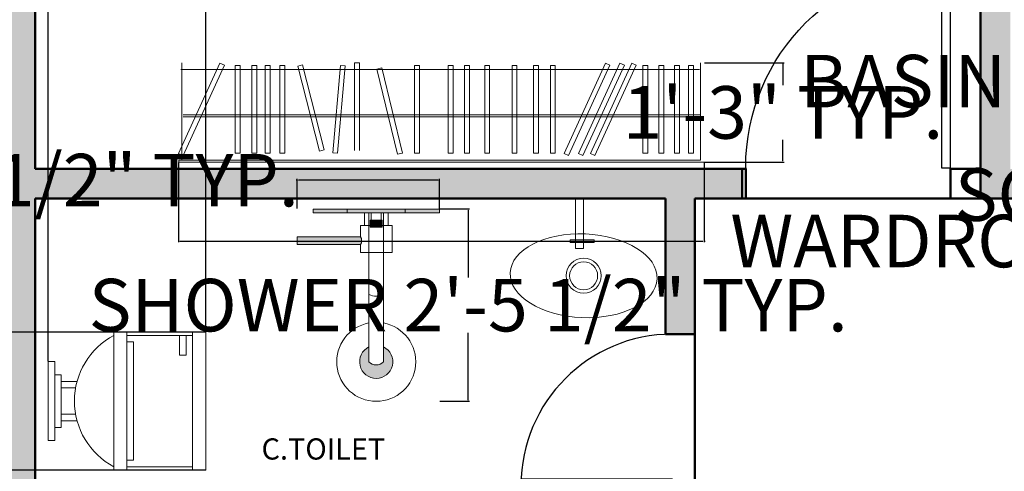
# Model space of a CAD drawing. Units: inches. Extents: x 22042254 to 25404563, y 17568978 to 17626777.
# Tile 39 of 45: x 22179790 to 22179940, y 17626539 to 17626607. Entities that reach past the tile are written whole.
import ezdxf

# ---------------------------------------------------------------- set-up
doc = ezdxf.new("R2010")
doc.units = ezdxf.units.IN
doc.header["$MEASUREMENT"] = 0
for name, color, linetype, lineweight in [('A-ANNO-DIMS', 2, 'Continuous', 18), ('A-AREA-IDEN', 7, 'Continuous', 18), ('A-WALL-PATT', 244, 'Continuous', 13), ('closet', 252, 'Continuous', 18), ('doors', 4, 'Continuous', 25), ('PLUMBING FIXTURES', 9, 'Continuous', 18), ('walls', 252, 'Continuous', 50)]:
    doc.layers.add(name, color=color, linetype=linetype, lineweight=lineweight)
doc.styles.get("Standard").update_dxf_attribs({"font": 'arial.ttf'})
doc.dimstyles.get("Standard").update_dxf_attribs({"dimtxt": 8, "dimasz": 0.18, "dimexe": 0.18, "dimexo": 0.0625, "dimgap": 0.09, "dimtad": 0, "dimtih": 1, "dimtoh": 1, "dimzin": 0, "dimdsep": 46, "dimlunit": 3, "dimtxsty": 'Standard', "dimcen": 0.09, "dimadec": 0, "dimazin": 0, "dimtfac": 1, "dimtofl": 0, "dimtmove": 0, "dimatfit": 3, "dimfxl": 1, "dimtolj": 1, "dimtzin": 0, "dimarcsym": 0})

# ---------------------------------------------------------------- blocks, each defined once
blk = doc.blocks.new('O.H SHOWER-PL')
at = {"layer": 'PLUMBING FIXTURES'}
for points in [[(-1.838, 0), (-1.838, -0.25), (1.838, -0.25), (1.838, 0)], [(0.461, -8.724), (0.461, -9.667, -0.422337), (-0.461, -9.667), (-0.461, -8.724, 4.325472)]]:
    blk.add_hatch(color=256, dxfattribs=at).paths.add_polyline_path(points)
for p, q in [((-1.838, 0), (-1.838, -0.25)), ((1.838, 0), (-1.838, 0)), ((1.838, 0), (1.838, -0.25)), ((1.838, -0.25), (-1.838, -0.25)), ((-0.461, -0.25), (-0.461, -9.667)), ((0.461, -0.25), (0.461, -9.667))]:
    blk.add_line(p, q, dxfattribs=at)
for centre, radius, start, end in [((0, -4.479), 1.033, 243.52996, 296.47004), ((0, -9.667), 2.501, 100.61004, 79.38997), ((0, -9.667), 1.049, 116.03487, 63.96515), ((0, -9.219), 0.643, 224.20776, 315.79224)]:
    blk.add_arc(centre, radius, start, end, dxfattribs=at)
blk = doc.blocks.new('DIVERTER-PL')
at = {"layer": 'PLUMBING FIXTURES'}
for points in [[(4, 0), (-4, 0), (-4, -0.25), (4, -0.25)], [(0.375, -1.144), (0.375, -0.704), (-0.375, -0.704), (-0.375, -1.144)], [(1, -1.751, 0.30818), (1, -2.251), (5, -2.251), (5, -1.751)]]:
    blk.add_hatch(color=256, dxfattribs=at).paths.add_polyline_path(points)
for p, q in [((-4, 0), (-4, -0.25)), ((-4, 0), (4, 0)), ((4, 0), (4, -0.25)), ((-4, -0.25), (4, -0.25)), ((-4, -0.25), (4, -0.25)), ((-0.75, -0.25), (-0.75, -1.05)), ((-0.318, -0.704), (-0.318, -0.25)), ((0.318, -0.704), (0.318, -0.25)), ((0.75, -0.25), (0.75, -1.05)), ((-1, -1.05), (-0.375, -1.05)), ((-1, -1.05), (-1, -2.75)), ((-0.375, -0.704), (0.375, -0.704)), ((-0.375, -0.704), (-0.375, -1.144)), ((-0.375, -1.144), (0.375, -1.144)), ((0.375, -0.704), (0.375, -1.144)), ((0.375, -1.05), (1, -1.05)), ((1, -1.05), (1, -1.751)), ((1, -2.251), (1, -2.75)), ((-1, -2.75), (1, -2.75))]:
    blk.add_line(p, q, dxfattribs=at)
at = {"layer": 'PLUMBING FIXTURES', "ltscale": 12}
for p, q in [((1, -1.751), (5, -1.751)), ((5, -2.251), (5, -1.751)), ((1, -2.251), (5, -2.251))]:
    blk.add_line(p, q, dxfattribs=at)
at = {"layer": 'PLUMBING FIXTURES'}
blk.add_arc((1.367, -2.001), 0.444, 145.74346, 214.25654, dxfattribs=at)
blk = doc.blocks.new('A$C7F153053')
at = {"layer": 'PLUMBING FIXTURES', "xscale": -1, "rotation": 270}
for name in ['DIVERTER-PL', 'O.H SHOWER-PL']:
    blk.add_blockref(name, (12.166, 4), dxfattribs=at)
blk = doc.blocks.new('closet')
at = {"layer": 'closet'}
for p, q in [((-0.71, -5.58), (5.59, 8.19)), ((6.27, 7.88), (-0.04, -5.89)), ((5.59, 8.19), (6.27, 7.88)), ((7.92, 7.84), (8.68, 7.84)), ((7.92, 7.84), (7.92, -5.51)), ((8.68, 7.84), (8.68, -5.51)), ((10.44, 7.84), (11.2, 7.84)), ((10.44, 7.84), (10.44, -5.51)), ((11.2, 7.84), (11.2, -5.51)), ((12.45, 7.84), (13.21, 7.84)), ((12.45, 7.84), (12.45, -5.51)), ((13.21, 7.84), (13.21, -5.51)), ((14.71, 7.84), (15.47, 7.84)), ((14.71, 7.84), (14.71, -5.51)), ((15.47, 7.84), (15.47, -5.51)), ((17.44, 7.75), (18.17, 7.93)), ((17.44, 7.75), (20.73, -5.2)), ((18.17, 7.93), (21.46, -5.01)), ((23.92, 7.84), (22.75, -5.46)), ((24.67, 7.78), (23.51, -5.53)), ((23.92, 7.84), (24.67, 7.78)), ((26.09, 8.25), (26.09, -5.1)), ((26.84, 8.25), (26.84, -5.1)), ((35.23, 7.84), (35.23, -5.51)), ((35.99, 7.84), (35.99, -5.51)), ((40.33, 7.84), (40.33, -5.51)), ((41.08, 7.84), (41.08, -5.51)), ((42.85, 7.84), (42.85, -5.51)), ((43.61, 7.84), (43.61, -5.51)), ((45.9, 7.84), (45.9, -5.51)), ((46.65, 7.84), (46.65, -5.51)), ((50.07, 7.84), (50.07, -5.51)), ((50.82, 7.84), (50.82, -5.51)), ((53.32, 7.84), (53.32, -5.51)), ((54.08, 7.84), (54.08, -5.51)), ((55.9, 7.84), (55.9, -5.51)), ((56.65, 7.84), (56.65, -5.51)), ((57.99, -5.58), (64.3, 8.19)), ((64.97, 7.88), (58.67, -5.89)), ((60.19, -5.58), (66.49, 8.19)), ((67.17, 7.88), (60.87, -5.89)), ((62, -5.58), (68.3, 8.19)), ((68.98, 7.88), (62.67, -5.89)), ((69.96, 7.84), (69.96, -5.51)), ((70.72, 7.84), (70.72, -5.51)), ((72.43, 7.84), (72.43, -5.51)), ((73.19, 7.84), (73.19, -5.51)), ((74.82, 7.84), (74.82, -5.51)), ((75.57, 7.84), (75.57, -5.51)), ((76.94, 7.84), (76.94, -5.51)), ((77.69, 7.84), (77.69, -5.51)), ((-0.23, 7.39), (-0.23, -6.57)), ((29.49, 7.29), (32.64, -5.69)), ((30.22, 7.46), (33.37, -5.51)), ((56.23, 0.33), (0, 0.33)), ((56.2, 0), (0, 0)), ((56.2, 0), (78.76, 0)), ((56.23, 0.33), (78.76, 0.33)), ((-0.04, -5.89), (-0.71, -5.58)), ((21.46, -5.01), (20.73, -5.2)), ((23.51, -5.53), (22.75, -5.46)), ((33.37, -5.51), (32.64, -5.69)), ((35.99, -5.51), (35.23, -5.51)), ((41.08, -5.51), (40.33, -5.51)), ((43.61, -5.51), (42.85, -5.51)), ((46.65, -5.51), (45.9, -5.51)), ((50.82, -5.51), (50.07, -5.51)), ((54.08, -5.51), (53.32, -5.51)), ((56.65, -5.51), (55.9, -5.51)), ((58.67, -5.89), (57.99, -5.58)), ((60.87, -5.89), (60.19, -5.58)), ((62.67, -5.89), (62, -5.58)), ((70.72, -5.51), (69.96, -5.51)), ((73.19, -5.51), (72.43, -5.51)), ((75.57, -5.51), (74.82, -5.51)), ((77.69, -5.51), (76.94, -5.51))]:
    blk.add_line(p, q, dxfattribs=at)
blk = doc.blocks.new('rotated closet')
at = {"layer": 'closet'}
for p, q in [((26.32, 0.86), (27.07, 0.86)), ((29.72, -0.11), (30.45, 0.07)), ((35.46, 0.45), (36.22, 0.45)), ((40.56, 0.45), (41.31, 0.45)), ((43.08, 0.45), (43.84, 0.45)), ((46.13, 0.45), (46.88, 0.45)), ((50.3, 0.45), (51.05, 0.45)), ((53.56, 0.45), (54.31, 0.45)), ((56.13, 0.45), (56.88, 0.45)), ((64.53, 0.8), (65.2, 0.49)), ((66.72, 0.8), (67.4, 0.49)), ((68.53, 0.8), (69.21, 0.49)), ((70.19, 0.45), (70.95, 0.45)), ((72.66, 0.45), (73.42, 0.45)), ((75.05, 0.45), (75.81, 0.45)), ((77.17, 0.45), (77.92, 0.45)), ((78.99, 0), (78.99, -13.96)), ((8.91, -12.91), (8.15, -12.91)), ((11.43, -12.91), (10.67, -12.91)), ((13.44, -12.91), (12.68, -12.91)), ((15.7, -12.91), (14.94, -12.91)), ((-0.46, -14.27), (79.54, -14.27)), ((0, -13.96), (78.99, -13.96))]:
    blk.add_line(p, q, dxfattribs=at)
blk.add_blockref('closet', (0.23, -7.39), dxfattribs=at)
blk = doc.blocks.new('Toilet - Imperial')
for p, q in [((-10, 22), (-10, 12)), ((-10, 21), (-7, 21)), ((-7, 21), (-7, 20)), ((10, 12), (10, 22)), ((-7, 20), (-10, 20)), ((10.5, 12), (-10.5, 12)), ((-10.5, 10), (-10.5, 12)), ((9, 13), (-9, 13)), ((-9, 13), (-9, 12)), ((9, 12), (9, 13)), ((10.5, 12), (10.5, 10)), ((10.5, 10), (-10.5, 10)), ((-3, 4.4065), (-3, 2)), ((-2, 2), (-2, 4.1658)), ((2, 4.1658), (2, 2)), ((3, 2), (3, 4.4065)), ((4, 2), (-4, 2)), ((-4, 2), (-4, 1)), ((4, 1), (4, 2))]:
    blk.add_line(p, q)
for points in [[(10.5, 22), (10.5, 24), (-10.5, 24), (-10.5, 22)], [(6, 0), (6, 1), (-6, 1), (-6, 0)]]:
    blk.add_lwpolyline(points, close=True)
blk.add_arc((0, 15.3333), 11.3333, 208.0725, 331.9275)
blk = doc.blocks.new('*U24')
for p, q in [((0, 0), (0, -6)), ((40, 0), (40, -6))]:
    blk.add_line(p, q)
blk.add_lwpolyline([(0, 0), (0, 40), (1.75, 40), (1.75, 0)], close=True)
blk.add_arc((0, 0), 40, 0, 90)
blk = doc.blocks.new('BASIN-OVAL-WITH-TAP')
for p, q in [((-5.47, 1.62), (-5.47, -2.04)), ((-5.06, 1.61), (-5.47, 1.61)), ((-5.06, -2.04), (-5.06, 1.61)), ((-11.77, 0), (-4.13, 0)), ((-4.13, 0), (-4.13, -1.24)), ((-4.13, -1.24), (-11.77, -1.24)), ((-5.47, -2.04), (-5.06, -2.04))]:
    blk.add_line(p, q)
for radius in [2.67, 2.13, 2.13, 2.13]:
    blk.add_circle((0, 0), radius)
blk.add_ellipse((0, 0), major_axis=(-0.46, -11.19), ratio=0.56899)
blk = doc.blocks.new('*D42')
at = {"layer": 'A-ANNO-DIMS', "color": 0, "lineweight": -2, "transparency": 16777216}
for p, q in [((22179814.6, 17626585.75), (22179814.6, 17626573.62)), ((22179894.63, 17626585.75), (22179894.63, 17626573.62)), ((22179814.78, 17626573.8), (22179894.45, 17626573.8)), ((22179894.63, 17626573.8), (22179894.81, 17626573.8))]:
    blk.add_line(p, q, dxfattribs=at)
at = {"layer": 'A-ANNO-DIMS', "color": 0, "transparency": 16777216}
for points in [[(22179814.78, 17626573.83), (22179814.78, 17626573.77), (22179814.6, 17626573.8)], [(22179894.45, 17626573.83), (22179894.45, 17626573.77), (22179894.63, 17626573.8)]]:
    blk.add_solid(points, dxfattribs=at)
at = {"layer": 'Defpoints', "color": 0, "transparency": 16777216}
for p in [(22179814.6, 17626585.81), (22179894.63, 17626585.81), (22179894.63, 17626573.8)]:
    blk.add_point(p, dxfattribs=at)
at = {"layer": 'A-ANNO-DIMS', "color": 0, "transparency": 16777216, "insert": (22179953.9, 17626573.8), "char_height": 8, "attachment_point": 5}
blk.add_mtext('\\A1;WARDROBE 6\'-8" TYP.', dxfattribs=at)
blk = doc.blocks.new('*D43')
at = {"layer": 'A-ANNO-DIMS', "color": 0, "lineweight": -2, "transparency": 16777216}
for p, q in [((22179894.69, 17626600.94), (22179906.81, 17626600.94)), ((22179906.63, 17626600.76), (22179906.63, 17626597.55)), ((22179906.63, 17626585.99), (22179906.63, 17626589.2)), ((22179894.69, 17626585.81), (22179906.81, 17626585.81))]:
    blk.add_line(p, q, dxfattribs=at)
at = {"layer": 'A-ANNO-DIMS', "color": 0, "transparency": 16777216}
for points in [[(22179906.6, 17626600.76), (22179906.66, 17626600.76), (22179906.63, 17626600.94)], [(22179906.6, 17626585.99), (22179906.66, 17626585.99), (22179906.63, 17626585.81)]]:
    blk.add_solid(points, dxfattribs=at)
at = {"layer": 'Defpoints', "color": 0, "transparency": 16777216}
for p in [(22179894.63, 17626600.94), (22179906.63, 17626600.94), (22179894.63, 17626585.81)]:
    blk.add_point(p, dxfattribs=at)
at = {"layer": 'A-ANNO-DIMS', "color": 0, "transparency": 16777216, "insert": (22179906.63, 17626593.38), "char_height": 8, "attachment_point": 5}
blk.add_mtext('\\A1;1\'-3" TYP.', dxfattribs=at)
blk = doc.blocks.new('*D44')
at = {"layer": 'A-ANNO-DIMS', "color": 0, "lineweight": -2, "transparency": 16777216}
for p, q in [((22179854.38, 17626578.68), (22179858.89, 17626578.68)), ((22179858.71, 17626578.5), (22179858.71, 17626568.26)), ((22179858.71, 17626549.58), (22179858.71, 17626559.81)), ((22179854.38, 17626549.4), (22179858.89, 17626549.4))]:
    blk.add_line(p, q, dxfattribs=at)
at = {"layer": 'A-ANNO-DIMS', "color": 0, "transparency": 16777216}
for points in [[(22179858.68, 17626578.5), (22179858.74, 17626578.5), (22179858.71, 17626578.68)], [(22179858.68, 17626549.58), (22179858.74, 17626549.58), (22179858.71, 17626549.4)]]:
    blk.add_solid(points, dxfattribs=at)
at = {"layer": 'Defpoints', "color": 0, "transparency": 16777216}
for p in [(22179854.32, 17626578.68), (22179858.71, 17626578.68), (22179854.32, 17626549.4)]:
    blk.add_point(p, dxfattribs=at)
at = {"layer": 'A-ANNO-DIMS', "color": 0, "transparency": 16777216, "insert": (22179858.71, 17626564.04), "char_height": 8, "attachment_point": 5}
blk.add_mtext('\\A1;SHOWER 2\'-5 1/2" TYP.', dxfattribs=at)
blk = doc.blocks.new('*D45')
at = {"layer": 'A-ANNO-DIMS', "color": 0, "lineweight": -2, "transparency": 16777216}
for p, q in [((22179832.67, 17626583.07), (22179832.49, 17626583.07)), ((22179832.67, 17626578.74), (22179832.67, 17626583.25)), ((22179854.14, 17626583.07), (22179832.85, 17626583.07)), ((22179854.32, 17626578.74), (22179854.32, 17626583.25))]:
    blk.add_line(p, q, dxfattribs=at)
at = {"layer": 'A-ANNO-DIMS', "color": 0, "transparency": 16777216}
for points in [[(22179832.85, 17626583.1), (22179832.85, 17626583.04), (22179832.67, 17626583.07)], [(22179854.14, 17626583.1), (22179854.14, 17626583.04), (22179854.32, 17626583.07)]]:
    blk.add_solid(points, dxfattribs=at)
at = {"layer": 'Defpoints', "color": 0, "transparency": 16777216}
for p in [(22179832.67, 17626583.07), (22179832.67, 17626578.68), (22179854.32, 17626578.68)]:
    blk.add_point(p, dxfattribs=at)
at = {"layer": 'A-ANNO-DIMS', "color": 0, "transparency": 16777216, "insert": (22179799.07, 17626583.07), "char_height": 8, "attachment_point": 5}
blk.add_mtext('\\A1;1\'-9 1/2" TYP.', dxfattribs=at)
blk = doc.blocks.new('*D46')
at = {"layer": 'A-ANNO-DIMS', "color": 0, "lineweight": -2, "transparency": 16777216}
for p, q in [((22179959.69, 17626609.47), (22179963.21, 17626609.47)), ((22179963.03, 17626609.29), (22179963.03, 17626602.36)), ((22179963.03, 17626586.98), (22179963.03, 17626593.91)), ((22179959.69, 17626586.8), (22179963.21, 17626586.8))]:
    blk.add_line(p, q, dxfattribs=at)
at = {"layer": 'A-ANNO-DIMS', "color": 0, "transparency": 16777216}
for points in [[(22179963, 17626609.29), (22179963.06, 17626609.29), (22179963.03, 17626609.47)], [(22179963, 17626586.98), (22179963.06, 17626586.98), (22179963.03, 17626586.8)]]:
    blk.add_solid(points, dxfattribs=at)
at = {"layer": 'Defpoints', "color": 0, "transparency": 16777216}
for p in [(22179959.63, 17626609.47), (22179963.03, 17626609.47), (22179959.63, 17626586.8)]:
    blk.add_point(p, dxfattribs=at)
at = {"layer": 'A-ANNO-DIMS', "color": 0, "transparency": 16777216, "insert": (22179963.03, 17626598.14), "char_height": 8, "attachment_point": 5}
blk.add_mtext('\\A1;BASIN 1\'-10 1/2" TYP.', dxfattribs=at)
blk = doc.blocks.new('*D48')
at = {"layer": 'A-ANNO-DIMS', "color": 0, "lineweight": -2, "transparency": 16777216}
for p, q in [((22180038.35, 17626580.87), (22180038.17, 17626580.87)), ((22180038.35, 17626570.34), (22180038.35, 17626581.05)), ((22180108.78, 17626580.87), (22180038.53, 17626580.87)), ((22180108.96, 17626570.34), (22180108.96, 17626581.05))]:
    blk.add_line(p, q, dxfattribs=at)
at = {"layer": 'A-ANNO-DIMS', "color": 0, "transparency": 16777216}
for points in [[(22180038.53, 17626580.9), (22180038.53, 17626580.84), (22180038.35, 17626580.87)], [(22180108.78, 17626580.9), (22180108.78, 17626580.84), (22180108.96, 17626580.87)]]:
    blk.add_solid(points, dxfattribs=at)
at = {"layer": 'Defpoints', "color": 0, "transparency": 16777216}
for p in [(22180038.35, 17626580.87), (22180038.35, 17626570.27), (22180108.96, 17626570.27)]:
    blk.add_point(p, dxfattribs=at)
at = {"layer": 'A-ANNO-DIMS', "color": 0, "transparency": 16777216, "insert": (22179984.52, 17626580.87), "char_height": 8, "attachment_point": 5}
blk.add_mtext('\\A1;SOFA 5\'-10 1/2" TYP.', dxfattribs=at)
blk = doc.blocks.new('*D60')
at = {"layer": 'A-ANNO-DIMS', "color": 0, "lineweight": -2, "transparency": 16777216}
for p, q in [((22179794.73, 17626555.5), (22179794.73, 17626772.16)), ((22179794.91, 17626771.98), (22179795.94, 17626771.98)), ((22179818.55, 17626771.98), (22179817.52, 17626771.98)), ((22179818.73, 17626560), (22179818.73, 17626772.16))]:
    blk.add_line(p, q, dxfattribs=at)
at = {"layer": 'A-ANNO-DIMS', "color": 0, "transparency": 16777216}
for points in [[(22179794.91, 17626772.01), (22179794.91, 17626771.95), (22179794.73, 17626771.98)], [(22179818.55, 17626772.01), (22179818.55, 17626771.95), (22179818.73, 17626771.98)]]:
    blk.add_solid(points, dxfattribs=at)
at = {"layer": 'Defpoints', "color": 0, "transparency": 16777216}
for p in [(22179818.73, 17626771.98), (22179818.73, 17626559.94), (22179794.73, 17626555.44)]:
    blk.add_point(p, dxfattribs=at)
at = {"layer": 'A-ANNO-DIMS', "color": 0, "transparency": 16777216, "insert": (22179806.73, 17626771.98), "char_height": 8, "attachment_point": 5}
blk.add_mtext('\\A1;2\'-0"', dxfattribs=at)
blk = doc.blocks.new('*D61')
at = {"layer": 'A-ANNO-DIMS', "color": 0, "lineweight": -2, "transparency": 16777216}
for p, q in [((22179818.67, 17626559.94), (22179727.35, 17626559.94)), ((22179727.53, 17626559.76), (22179727.53, 17626553.61)), ((22179727.53, 17626539.12), (22179727.53, 17626545.26)), ((22179818.67, 17626538.94), (22179727.35, 17626538.94))]:
    blk.add_line(p, q, dxfattribs=at)
at = {"layer": 'A-ANNO-DIMS', "color": 0, "transparency": 16777216}
for points in [[(22179727.5, 17626559.76), (22179727.56, 17626559.76), (22179727.53, 17626559.94)], [(22179727.5, 17626539.12), (22179727.56, 17626539.12), (22179727.53, 17626538.94)]]:
    blk.add_solid(points, dxfattribs=at)
at = {"layer": 'Defpoints', "color": 0, "transparency": 16777216}
for p in [(22179818.73, 17626559.94), (22179727.53, 17626538.94), (22179818.73, 17626538.94)]:
    blk.add_point(p, dxfattribs=at)
at = {"layer": 'A-ANNO-DIMS', "color": 0, "transparency": 16777216, "insert": (22179727.53, 17626549.44), "char_height": 8, "attachment_point": 5}
blk.add_mtext('\\A1;1\'-9"', dxfattribs=at)

msp = doc.modelspace()

# ---------------------------------------------------------------- hatches: boundary and pattern name
at = {"layer": 'A-WALL-PATT'}
h = msp.add_hatch(color=256, dxfattribs=at)
h.dxf.hatch_style = 1
h.paths.add_polyline_path([(22179792.734, 17626580.28), (22179888.734, 17626580.28), (22179888.734, 17626559.623), (22179893.234, 17626559.623), (22179893.234, 17626580.28), (22179900.438, 17626580.28), (22179900.438, 17626584.78), (22179792.734, 17626584.78), (22179792.734, 17626728.78), (22180134.734, 17626728.78), (22180134.734, 17626584.78), (22180035.602, 17626584.78), (22180004.432, 17626584.78), (22180001.734, 17626584.78), (22180001.734, 17626580.28), (22180134.734, 17626580.28), (22180134.734, 17626404.28), (22180064.487, 17626404.28), (22180064.487, 17626399.78), (22180134.734, 17626399.78), (22180134.734, 17626197.78), (22180143.734, 17626197.78), (22180143.734, 17626737.78), (22179783.734, 17626737.78), (22179783.734, 17626197.78), (22179792.734, 17626197.78), (22179792.734, 17626394.78), (22179936.734, 17626394.78), (22179936.734, 17626383.208), (22179941.234, 17626383.208), (22179941.234, 17626532.28), (22179927.066, 17626532.28), (22179927.066, 17626527.78), (22179928.072, 17626527.78), (22179936.734, 17626527.78), (22179936.734, 17626403.78), (22179792.734, 17626403.78), (22179792.734, 17626527.78), (22179905.094, 17626527.78), (22179905.094, 17626532.28), (22179792.734, 17626532.28)])
h = msp.add_hatch(color=256, dxfattribs=at)
h.dxf.hatch_style = 1
h.paths.add_polyline_path([(22179941.234, 17626676.28), (22179997.234, 17626676.28), (22179997.234, 17626614.838), (22180001.734, 17626614.838), (22180001.734, 17626680.78), (22179936.734, 17626680.78), (22179936.734, 17626617.551), (22179936.734, 17626580.28), (22179941.234, 17626580.28), (22180001.734, 17626580.28), (22180001.734, 17626591.815), (22179997.234, 17626591.815), (22179997.234, 17626584.78), (22179941.234, 17626584.78)])

# ---------------------------------------------------------------- linework, layer by layer
at = {"layer": 'closet'}
for p, q in [((22179815.082, 17626600.933), (22179815.082, 17626586.123)), ((22179894.071, 17626586.123), (22179894.071, 17626600.933)), ((22179893.948, 17626599.905), (22179814.959, 17626599.905)), ((22179814.625, 17626585.808), (22179814.625, 17626586.123)), ((22179814.625, 17626586.123), (22179815.082, 17626586.123)), ((22179814.625, 17626585.808), (22179894.625, 17626585.808)), ((22179814.625, 17626585.808), (22179894.625, 17626585.808)), ((22179814.625, 17626585.808), (22179894.625, 17626585.808)), ((22179815.082, 17626586.123), (22179892.427, 17626586.123)), ((22179815.082, 17626586.123), (22179894.071, 17626586.123)), ((22179891.967, 17626585.808), (22179894.068, 17626585.808)), ((22179891.967, 17626585.808), (22179894.068, 17626585.808)), ((22179814.503, 17626584.78), (22179894.503, 17626584.78))]:
    msp.add_line(p, q, dxfattribs=at)
at = {"layer": 'walls'}
for p, q in [((22179792.734, 17626584.78), (22179792.734, 17626728.78)), ((22179936.734, 17626580.28), (22179936.734, 17626728.78)), ((22179792.734, 17626584.78), (22179900.959, 17626584.78)), ((22179900.438, 17626584.78), (22179900.438, 17626580.28)), ((22179900.959, 17626584.78), (22179900.959, 17626580.28)), ((22179932.13, 17626584.78), (22179936.734, 17626584.78)), ((22179932.13, 17626584.78), (22179932.13, 17626580.28)), ((22179792.734, 17626580.28), (22179888.734, 17626580.28)), ((22179792.734, 17626580.28), (22179888.734, 17626580.28)), ((22179792.734, 17626532.28), (22179792.734, 17626580.28)), ((22179888.734, 17626559.599), (22179888.734, 17626580.28)), ((22179893.234, 17626580.28), (22179941.234, 17626580.28)), ((22179893.234, 17626580.28), (22180134.734, 17626580.28)), ((22179893.234, 17626532.28), (22179893.234, 17626580.28)), ((22179888.734, 17626559.599), (22179893.234, 17626559.623)), ((22179888.734, 17626559.623), (22179893.234, 17626559.623)), ((22179888.734, 17626559.599), (22179888.734, 17626559.623)), ((22179893.234, 17626559.623), (22179893.234, 17626536.599))]:
    msp.add_line(p, q, dxfattribs=at)

# ---------------------------------------------------------------- block references
at = {"layer": 'closet'}
msp.add_blockref('rotated closet', (22179815.082, 17626600.083), dxfattribs=at)
at = {"layer": 'doors', "xscale": -0.7792671805443983, "yscale": 0.7792671805443983, "zscale": 0.7792671805443983}
msp.add_blockref('*U24', (22179932.13, 17626584.955), dxfattribs=at)
at = {"layer": 'doors', "xscale": 0.5755769432943251, "yscale": 0.5755769432943251, "zscale": 0.5755769432943251, "rotation": 90}
msp.add_blockref('*U24', (22179889.78, 17626536.599), dxfattribs=at)
at = {"layer": 'PLUMBING FIXTURES'}
for name, p, rotation in [('BASIN-OVAL-WITH-TAP', (22179876.281, 17626568.508), 269.9999995201874), ('Toilet - Imperial', (22179794.734, 17626549.436), 270)]:
    msp.add_blockref(name, p, dxfattribs=dict(at, rotation=rotation))
at = {"layer": 'PLUMBING FIXTURES', "xscale": 2.406230429091579, "yscale": 2.406230429091579, "zscale": 2.406230429091579, "rotation": 90}
msp.add_blockref('A$C7F153053', (22179854.322, 17626549.401), dxfattribs=at)

# ---------------------------------------------------------------- texts
at = {"layer": 'A-AREA-IDEN'}
msp.add_text('C.TOILET', height=3.2253, dxfattribs=at).set_placement((22179827.231, 17626540.53))

# ---------------------------------------------------------------- dimensions: what is measured, and where the dimension line sits
at = {"layer": 'A-ANNO-DIMS'}
dim = msp.add_linear_dim(base=(22179818.734, 17626771.98), p1=(22179794.734, 17626555.436), p2=(22179818.734, 17626559.936), dimstyle='Standard', override={"dimdec": 1, "dimlfac": 1, "dimrnd": 0, "dimzin": 1, "dimdsep": 46, "dimlunit": 4, "dimfrac": 2}, dxfattribs=at)
dim.commit()
dim.dimension.update_dxf_attribs({"geometry": '*D60', "text_midpoint": (22179806.734, 17626771.98)})
for base, p1, p2, angle, text, picture, middle in [((22179963.03, 17626609.475), (22179959.629, 17626586.798), (22179959.629, 17626609.475), 90, 'BASIN <> TYP.', '*D46', (22179963.03, 17626598.136)), ((22179906.629, 17626600.942), (22179894.625, 17626585.808), (22179894.625, 17626600.942), 90, '<> TYP.', '*D43', (22179906.629, 17626593.375)), ((22180038.35, 17626580.865), (22180108.959, 17626570.274), (22180038.35, 17626570.274), 180, 'SOFA <> TYP.', '*D48', (22179984.522, 17626580.865)), ((22179832.666, 17626583.067), (22179854.322, 17626578.675), (22179832.666, 17626578.675), 180, '<> TYP.', '*D45', (22179799.07, 17626583.067)), ((22179858.713, 17626578.675), (22179854.322, 17626549.396), (22179854.322, 17626578.675), 90, 'SHOWER <> TYP.', '*D44', (22179858.713, 17626564.036))]:
    dim = msp.add_linear_dim(base=base, p1=p1, p2=p2, angle=angle, text=text, dimstyle='Standard', override={"dimdec": 1, "dimlfac": 1, "dimrnd": 0, "dimzin": 1, "dimdsep": 46, "dimlunit": 4, "dimfrac": 2}, dxfattribs=at)
    dim.commit()
    dim.dimension.update_dxf_attribs({"geometry": picture, "text_midpoint": middle})
dim = msp.add_linear_dim(base=(22179894.625, 17626573.805), p1=(22179814.602, 17626585.808), p2=(22179894.625, 17626585.808), text='WARDROBE <> TYP.', dimstyle='Standard', override={"dimdec": 1, "dimlfac": 1, "dimrnd": 0, "dimzin": 1, "dimdsep": 46, "dimlunit": 4, "dimfrac": 2}, dxfattribs=at)
dim.commit()
dim.dimension.update_dxf_attribs({"geometry": '*D42', "text_midpoint": (22179953.902, 17626573.805)})
dim = msp.add_linear_dim(base=(22179727.534, 17626538.936), p1=(22179818.734, 17626559.936), p2=(22179818.734, 17626538.936), angle=90, dimstyle='Standard', override={"dimdec": 1, "dimlfac": 1, "dimrnd": 0, "dimzin": 1, "dimdsep": 46, "dimlunit": 4, "dimfrac": 2}, dxfattribs=at)
dim.commit()
dim.dimension.update_dxf_attribs({"geometry": '*D61', "text_midpoint": (22179727.534, 17626549.436)})

doc.saveas('drawing.dxf')
